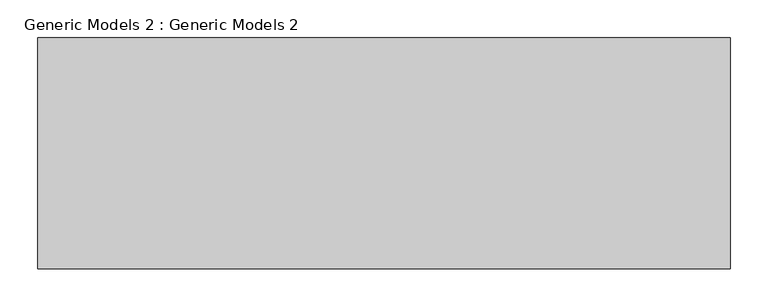
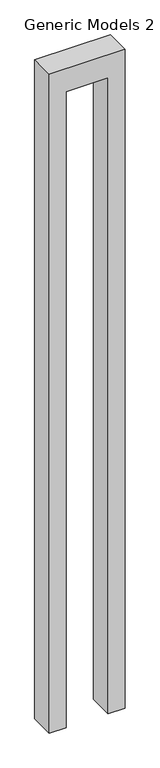
"""IFC4 building model written with IfcOpenShell, lengths in millimetres: proxy geometry, Generic Models 2 : Generic Models 2."""

from ifc_helpers import new_model, si_unit, frame, origin, place, context, project, spatial, polyline, outline, extrude, source, transform, mapped, element, save


def generic_models_2_generic_models_2_975c2898(model_context):
    return source(origin(), model_context, "Body", "SweptSolid", [
        extrude(outline(polyline([(8419.1061715, -8345.5126504), (8419.1061715, -9259.9126504), (0.0, -9259.9126504), (0.0, -9056.7126504), (8126.5892965, -9056.7126504), (8126.5892965, -8548.7126504), (0.0, -8548.7126504), (0.0, -8345.5126504), (8419.1061715, -8345.5126504)])), frame((0.0, -4355.271143, 0.0), z_axis=(0.0, 1.0, 0.0), x_axis=(0.0, 0.0, 1.0)), (0.0, 0.0, 1.0), 304.8),
    ])


if __name__ == "__main__":
    model = new_model("IFC4")
    model_context = context("Model", 3, world=origin())
    ifc_project = project(units=[si_unit("LENGTHUNIT", "METRE", prefix="MILLI")], contexts=[model_context])
    site = spatial("IfcSite", under=ifc_project)
    building = spatial("IfcBuilding", under=site)
    placement = place(None, origin())
    generic_models_2_generic_models_2_shape = generic_models_2_generic_models_2_975c2898(model_context)
    element("IfcBuildingElementProxy", 1, Name="Generic Models 2 : Generic Models 2", ObjectType="Generic Models 2 : Generic Models 2", at=placement, inside=building, context=model_context, shape_type="MappedRepresentation", body=[
        mapped(generic_models_2_generic_models_2_shape, transform((0.0, 0.0, 0.0), x_axis=(1.0, 0.0, 0.0), y_axis=(0.0, 1.0, 0.0), z_axis=(0.0, 0.0, 1.0))),
    ])
    save(model, "model.ifc")
